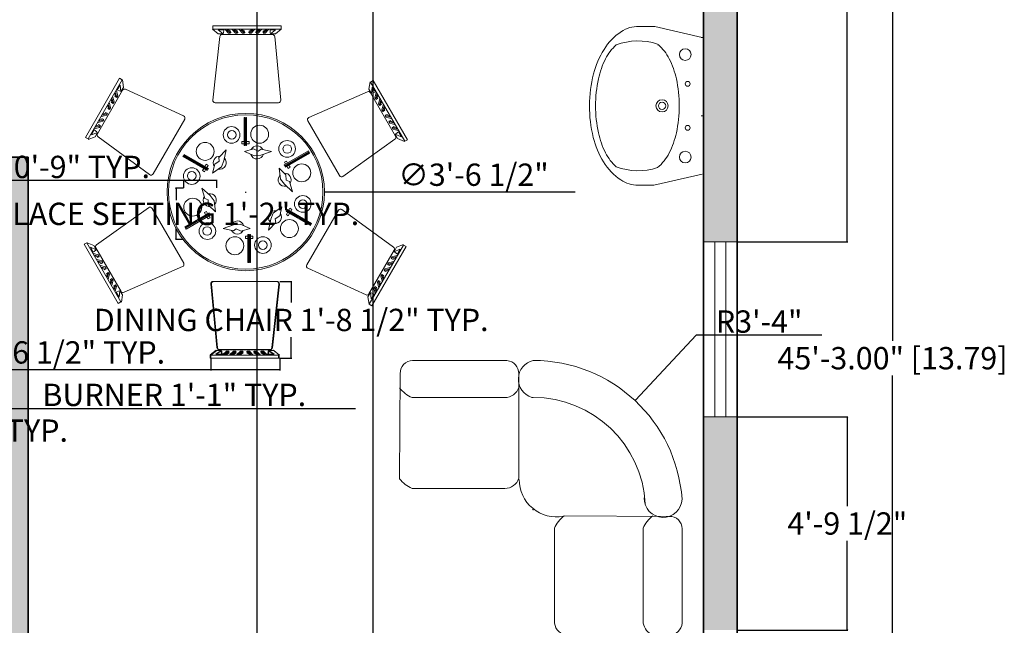
# Model space of a CAD drawing. Units: inches. Extents: x 2322 to 2932, y 142 to 762.
# Tile 6 of 7: x 2609 to 2874, y 376 to 538. Entities that reach past the tile are written whole.
import ezdxf

# ---------------------------------------------------------------- set-up
doc = ezdxf.new("R2010")
doc.units = ezdxf.units.IN
doc.header["$MEASUREMENT"] = 0
for name, color, linetype, lineweight in [('A-ANNO-DIMS', 2, 'Continuous', 18), ('A-FLOR-FIXT', 9, 'Continuous', 18), ('A-GLAZ', 4, 'Continuous', 18), ('A-WALL', 7, 'Continuous', 35)]:
    doc.layers.add(name, color=color, linetype=linetype, lineweight=lineweight)
doc.layers.add('A-WALL-PATT', color=40, linetype='Continuous', lineweight=13, true_color=0xf8d731)
doc.layers.add('Furniture', color=7, linetype='Continuous', lineweight=15, true_color=0xffffff)
doc.styles.get("Standard").update_dxf_attribs({"font": 'italic8.shx'})
doc.dimstyles.get("Standard").update_dxf_attribs({"dimtxt": 6, "dimasz": 0.15, "dimexe": 0.18, "dimexo": 0.0625, "dimgap": 0.09, "dimtad": 1, "dimtih": 1, "dimtoh": 1, "dimzin": 0, "dimdsep": 46, "dimlunit": 3, "dimtxsty": 'Standard', "dimblk": 'CLOSEDBLANK', "dimcen": 0.09, "dimclrd": 3, "dimclre": 1, "dimclrt": 6, "dimadec": 0, "dimazin": 0, "dimtfac": 1, "dimtofl": 0, "dimtmove": 0, "dimatfit": 3, "dimldrblk": 'DOT', "dimfxl": 1, "dimtolj": 1, "dimtzin": 0, "dimarcsym": 0})

# ---------------------------------------------------------------- blocks, each defined once
blk = doc.blocks.new('_ClosedBlank')
at = {"color": 0, "linetype": 'ByBlock', "lineweight": -2}
for p, q in [((-1, 0.2), (0, 0)), ((-1, 0.2), (-1, -0.2)), ((0, 0), (-1, -0.2))]:
    blk.add_line(p, q, dxfattribs=at)
blk = doc.blocks.new('*D3')
at = {"layer": 'A-ANNO-DIMS', "color": 0, "lineweight": -2, "transparency": 16777216}
for p, q in [((2802.13, 718.82), (2844.02, 718.82)), ((2843.84, 718.67), (2843.84, 451.98)), ((2843.84, 175.97), (2843.84, 442.66)), ((2802.13, 175.82), (2844.02, 175.82))]:
    blk.add_line(p, q, dxfattribs=at)
at = {"layer": 'Defpoints', "color": 0, "transparency": 16777216}
for p in [(2802.06, 718.82), (2802.06, 175.82), (2843.84, 175.82)]:
    blk.add_point(p, dxfattribs=at)
at = {"layer": 'A-ANNO-DIMS', "color": 0, "lineweight": -2, "transparency": 16777216, "xscale": 0.15, "yscale": 0.15, "zscale": 0.15}
for p, rotation in [((2843.84, 718.82), 90), ((2843.84, 175.82), 270)]:
    blk.add_blockref('_ClosedBlank', p, dxfattribs=dict(at, rotation=rotation))
at = {"layer": 'A-ANNO-DIMS', "color": 0, "transparency": 16777216, "insert": (2843.84, 447.32), "char_height": 6, "attachment_point": 5}
blk.add_mtext('\\A1;45\'-3.00" [13.79]', dxfattribs=at)
blk = doc.blocks.new('_Dot')
at = {"color": 0, "linetype": 'ByBlock', "lineweight": -2}
blk.add_line((-0.5, 0), (-1, 0), dxfattribs=at)
at = {"color": 0, "linetype": 'ByBlock', "const_width": 0.5}
blk.add_lwpolyline([(-0.25, 0, 1), (0.25, 0, 1)], format="xyb", close=True, dxfattribs=at)
blk = doc.blocks.new('WINDOW-47X9')
for p, q in [((47, 9), (0, 9)), ((0, 9), (0, 0)), ((47, 0), (47, 9)), ((0, 6), (47, 6)), ((0, 3), (47, 3)), ((0, 0), (47, 0))]:
    blk.add_line(p, q)
blk = doc.blocks.new('CHAIR-DINING')
for p, q in [((0, 19.73, 3.57), (1.57, 18.47, 3.57)), ((0.13, 20.61, 3.57), (0.13, 19.79, 3.57)), ((18.48, 20.61, 3.57), (0.13, 20.61, 3.57)), ((0.13, 19.79, 3.57), (18.48, 19.79, 3.57)), ((1.51, 19.54, 3.57), (3.02, 19.6, 3.57)), ((2.89, 18.53, 3.57), (1.51, 19.54, 3.57)), ((1.57, 18.47, 3.57), (2.89, 18.53, 3.57)), ((3.02, 19.6, 3.57), (2.95, 18.72, 3.57)), ((3.39, 19.66, 3.57), (4.34, 18.72, 3.57)), ((3.9, 19.6, 3.57), (4.27, 19.6, 3.57)), ((4.84, 18.72, 3.57), (3.9, 19.6, 3.57)), ((4.27, 19.6, 3.57), (4.71, 19.22, 3.57)), ((4.34, 18.72, 3.57), (4.84, 18.72, 3.57)), ((4.71, 19.22, 3.57), (4.84, 19.35, 3.57)), ((4.84, 19.35, 3.57), (4.9, 18.78, 3.57)), ((5.28, 19.66, 3.57), (6.22, 18.72, 3.57)), ((5.78, 19.6, 3.57), (6.16, 19.6, 3.57)), ((6.73, 18.72, 3.57), (5.78, 19.6, 3.57)), ((6.16, 19.6, 3.57), (6.6, 19.22, 3.57)), ((6.22, 18.72, 3.57), (6.73, 18.72, 3.57)), ((6.6, 19.22, 3.57), (6.73, 19.35, 3.57)), ((6.73, 19.35, 3.57), (6.79, 18.78, 3.57)), ((7.17, 19.66, 3.57), (8.11, 18.72, 3.57)), ((7.67, 19.6, 3.57), (8.05, 19.6, 3.57)), ((8.61, 18.72, 3.57), (7.67, 19.6, 3.57)), ((8.05, 19.6, 3.57), (8.49, 19.22, 3.57)), ((8.11, 18.72, 3.57), (8.61, 18.72, 3.57)), ((8.49, 19.22, 3.57), (8.61, 19.35, 3.57)), ((8.61, 19.35, 3.57), (8.67, 18.78, 3.57)), ((9.87, 19.35, 3.57), (9.81, 18.78, 3.57)), ((9.87, 18.72, 3.57), (10.81, 19.6, 3.57)), ((9.99, 19.22, 3.57), (9.87, 19.35, 3.57)), ((10.37, 18.72, 3.57), (9.87, 18.72, 3.57)), ((10.43, 19.6, 3.57), (9.99, 19.22, 3.57)), ((11.31, 19.66, 3.57), (10.37, 18.72, 3.57)), ((10.81, 19.6, 3.57), (10.43, 19.6, 3.57)), ((11.75, 19.35, 3.57), (11.69, 18.78, 3.57)), ((11.75, 18.72, 3.57), (12.7, 19.6, 3.57)), ((11.88, 19.22, 3.57), (11.75, 19.35, 3.57)), ((12.26, 18.72, 3.57), (11.75, 18.72, 3.57)), ((12.32, 19.6, 3.57), (11.88, 19.22, 3.57)), ((13.2, 19.66, 3.57), (12.26, 18.72, 3.57)), ((12.7, 19.6, 3.57), (12.32, 19.6, 3.57)), ((13.64, 19.35, 3.57), (13.58, 18.78, 3.57)), ((13.64, 18.72, 3.57), (14.58, 19.6, 3.57)), ((13.77, 19.22, 3.57), (13.64, 19.35, 3.57)), ((14.14, 18.72, 3.57), (13.64, 18.72, 3.57)), ((14.21, 19.6, 3.57), (13.77, 19.22, 3.57)), ((15.09, 19.66, 3.57), (14.14, 18.72, 3.57)), ((14.58, 19.6, 3.57), (14.21, 19.6, 3.57)), ((15.46, 19.6, 3.57), (15.53, 18.72, 3.57)), ((16.97, 19.54, 3.57), (15.46, 19.6, 3.57)), ((15.59, 18.53, 3.57), (16.97, 19.54, 3.57)), ((16.91, 18.47, 3.57), (15.59, 18.53, 3.57)), ((18.48, 19.73, 3.57), (16.91, 18.47, 3.57)), ((18.48, 19.79, 3.57), (18.48, 20.61, 3.57)), ((0.08, 0.7, 3.57), (1.95, 17.78, 3.57)), ((2.58, 18.34, 3.57), (16.09, 18.34, 3.57)), ((16.71, 17.78, 3.57), (18.35, 0.69, 3.57)), ((17.72, 0, 3.57), (0.7, 0, 3.57))]:
    blk.add_line(p, q)
for centre, start, end in [((2.58, 17.72, 3.57), 90, 173.7428), ((16.09, 17.72, 3.57), 5.4801, 90), ((0.7, 0.63, 3.57), 173.7428, 270), ((17.72, 0.63, 3.57), 270, 5.4801)]:
    blk.add_arc(centre, 0.629, start, end)
blk = doc.blocks.new('DINING-PLACE-SETTING')
for p, q in [((8.13, 10.96, 7.15), (1.62, 7.2, 7.15)), ((1.74, 6.99, 7.15), (8.25, 10.75, 7.15)), ((8.25, 10.75, 7.15), (8.13, 10.96, 7.15)), ((2.23, 8.25, 7.15), (1.7, 7.95, 7.15)), ((1.7, 7.95, 7.15), (2.01, 7.42, 7.15)), ((8.35, 10.57, 7.15), (1.84, 6.81, 7.15)), ((1.96, 6.61, 7.15), (8.47, 10.37, 7.15)), ((2.54, 7.72, 7.15), (2.23, 8.25, 7.15)), ((8.47, 10.37, 7.15), (8.35, 10.57, 7.15)), ((2.07, 4.55, 7.15), (0.25, 6.3, 7.15)), ((0.25, 6.3, 7.15), (0.59, 3.36, 7.15)), ((1.62, 7.2, 7.15), (1.74, 6.99, 7.15)), ((1.84, 6.81, 7.15), (1.96, 6.61, 7.15)), ((2.12, 7.22, 7.15), (2.23, 7.03, 7.15)), ((2.35, 6.83, 7.15), (2.68, 6.26, 7.15)), ((2.76, 7.34, 7.15), (2.65, 7.52, 7.15)), ((2.68, 6.26, 7.15), (3.21, 6.56, 7.15)), ((3.21, 6.56, 7.15), (2.88, 7.13, 7.15)), ((0.59, 3.36, 7.15), (1.66, 1.99, 7.15)), ((2.19, 3.11, 7.15), (2.07, 4.55, 7.15)), ((3.08, 2.74, 7.15), (2.19, 3.11, 7.15)), ((3.88, 0, 7.15), (3.08, 2.74, 7.15)), ((1.66, 1.99, 7.15), (3.88, 0, 7.15))]:
    blk.add_line(p, q)
for centre, radius in [((2.41, 11.52, 7.15), 2.24), ((2.46, 11.49, 7.15), 1.16), ((6.34, 5.08, 7.15), 2.41)]:
    blk.add_circle(centre, radius)
for start, end in [(137.0611, 284.0662), (326.6641, 94.1442)]:
    blk.add_arc((1.75, 3.22, 7.15), 1.75, start, end)
blk = doc.blocks.new('SECTIONAL-SEAT')
for p, q in [((30.86, 31.9), (2.62, 32.04)), ((0, 28.69), (0, 3.79)), ((23.85, 28.69), (23.85, 3.79)), ((34.36, 3.2), (34.36, 28.55)), ((2.77, 0), (30.86, 0))]:
    blk.add_line(p, q)
for centre, radius, start, end in [((7.53, 25.51), 8.17, 126.8838, 157.0502), ((31.38, 25.51), 8.17, 126.8838, 157.0502), ((31, 28.55), 3.35, 0, 92.4088), ((3.98, 3.79), 3.98, 180, 252.2888), ((27.83, 3.79), 3.98, 180, 244.0743), ((30.86, 3.51), 3.51, 270, 355.0498)]:
    blk.add_arc(centre, radius, start, end)
blk = doc.blocks.new('*D30')
at = {"layer": 'A-ANNO-DIMS', "color": 1, "lineweight": -2, "transparency": 16777216}
for p, q in [((2679.23, 467.9), (2682.44, 467.9)), ((2679.23, 447.3), (2682.44, 447.3))]:
    blk.add_line(p, q, dxfattribs=at)
at = {"layer": 'A-ANNO-DIMS', "color": 3, "lineweight": -2, "transparency": 16777216}
for p, q in [((2682.26, 467.75), (2682.26, 462.26)), ((2682.26, 447.45), (2682.26, 452.94))]:
    blk.add_line(p, q, dxfattribs=at)
at = {"layer": 'Defpoints', "color": 0, "transparency": 16777216}
for p in [(2679.17, 467.9), (2679.17, 447.3), (2682.26, 447.3)]:
    blk.add_point(p, dxfattribs=at)
at = {"layer": 'A-ANNO-DIMS', "color": 3, "lineweight": -2, "transparency": 16777216, "xscale": 0.15, "yscale": 0.15, "zscale": 0.15}
for p, rotation in [((2682.26, 467.9), 90), ((2682.26, 447.3), 270)]:
    blk.add_blockref('_ClosedBlank', p, dxfattribs=dict(at, rotation=rotation))
at = {"layer": 'A-ANNO-DIMS', "color": 6, "transparency": 16777216, "insert": (2682.26, 457.6), "char_height": 6, "attachment_point": 5}
blk.add_mtext('\\A1;DINING CHAIR 1\'-8 1/2" TYP.', dxfattribs=at)
blk = doc.blocks.new('*D31')
at = {"layer": 'A-ANNO-DIMS', "color": 1, "lineweight": -2, "transparency": 16777216}
for p, q in [((2660.69, 447.24), (2660.69, 444.03)), ((2679.17, 447.24), (2679.17, 444.03))]:
    blk.add_line(p, q, dxfattribs=at)
at = {"layer": 'A-ANNO-DIMS', "color": 3, "lineweight": -2, "transparency": 16777216}
for p, q in [((2660.69, 444.21), (2585.5, 444.21)), ((2679.02, 444.21), (2660.84, 444.21))]:
    blk.add_line(p, q, dxfattribs=at)
at = {"layer": 'Defpoints', "color": 0, "transparency": 16777216}
for p in [(2660.69, 447.3), (2679.17, 447.3), (2660.69, 444.21)]:
    blk.add_point(p, dxfattribs=at)
at = {"layer": 'A-ANNO-DIMS', "color": 3, "lineweight": -2, "transparency": 16777216, "xscale": 0.15, "yscale": 0.15, "zscale": 0.15, "rotation": 180}
blk.add_blockref('_ClosedBlank', (2660.69, 444.21), dxfattribs=at)
at = {"layer": 'A-ANNO-DIMS', "color": 3, "lineweight": -2, "transparency": 16777216, "xscale": 0.15, "yscale": 0.15, "zscale": 0.15}
blk.add_blockref('_ClosedBlank', (2679.17, 444.21), dxfattribs=at)
at = {"layer": 'A-ANNO-DIMS', "color": 6, "transparency": 16777216, "insert": (2623.02, 448.87), "char_height": 6, "attachment_point": 5}
blk.add_mtext('\\A1;1\'-6 1/2" TYP.', dxfattribs=at)
blk = doc.blocks.new('*D32')
at = {"layer": 'A-ANNO-DIMS', "color": 1, "lineweight": -2, "transparency": 16777216}
for p, q in [((2653.34, 493), (2651.16, 493)), ((2653.34, 479.24), (2651.16, 479.24))]:
    blk.add_line(p, q, dxfattribs=at)
at = {"layer": 'A-ANNO-DIMS', "color": 3, "lineweight": -2, "transparency": 16777216}
for p, q in [((2651.34, 492.85), (2651.34, 489.78)), ((2651.34, 479.39), (2651.34, 482.46))]:
    blk.add_line(p, q, dxfattribs=at)
at = {"layer": 'Defpoints', "color": 0, "transparency": 16777216}
for p in [(2653.4, 493), (2651.34, 479.24), (2653.4, 479.24)]:
    blk.add_point(p, dxfattribs=at)
at = {"layer": 'A-ANNO-DIMS', "color": 3, "lineweight": -2, "transparency": 16777216, "xscale": 0.15, "yscale": 0.15, "zscale": 0.15}
for p, rotation in [((2651.34, 493), 90), ((2651.34, 479.24), 270)]:
    blk.add_blockref('_ClosedBlank', p, dxfattribs=dict(at, rotation=rotation))
at = {"layer": 'A-ANNO-DIMS', "color": 6, "transparency": 16777216, "insert": (2651.34, 486.12), "char_height": 6, "attachment_point": 5}
blk.add_mtext('\\A1;PLACE SETTING 1\'-2" TYP.', dxfattribs=at)
blk = doc.blocks.new('*D33')
at = {"layer": 'A-ANNO-DIMS', "color": 3, "lineweight": -2, "transparency": 16777216}
for p, q in [((2653.4, 495.07), (2598.79, 495.07)), ((2662.16, 495.07), (2653.55, 495.07))]:
    blk.add_line(p, q, dxfattribs=at)
at = {"layer": 'A-ANNO-DIMS', "color": 1, "lineweight": -2, "transparency": 16777216}
for p, q in [((2653.4, 493.07), (2653.4, 495.25)), ((2662.31, 493.07), (2662.31, 495.25))]:
    blk.add_line(p, q, dxfattribs=at)
at = {"layer": 'Defpoints', "color": 0, "transparency": 16777216}
for p in [(2653.4, 495.07), (2653.4, 493), (2662.31, 493)]:
    blk.add_point(p, dxfattribs=at)
at = {"layer": 'A-ANNO-DIMS', "color": 3, "lineweight": -2, "transparency": 16777216, "xscale": 0.15, "yscale": 0.15, "zscale": 0.15, "rotation": 180}
blk.add_blockref('_ClosedBlank', (2653.4, 495.07), dxfattribs=at)
at = {"layer": 'A-ANNO-DIMS', "color": 3, "lineweight": -2, "transparency": 16777216, "xscale": 0.15, "yscale": 0.15, "zscale": 0.15}
blk.add_blockref('_ClosedBlank', (2662.31, 495.07), dxfattribs=at)
at = {"layer": 'A-ANNO-DIMS', "color": 6, "transparency": 16777216, "insert": (2626.02, 498.73), "char_height": 6, "attachment_point": 5}
blk.add_mtext('\\A1;0\'-9" TYP.', dxfattribs=at)
blk = doc.blocks.new('*D42')
at = {"layer": 'A-ANNO-DIMS', "color": 1, "lineweight": -2, "transparency": 16777216}
for p, q in [((2589.15, 431.92), (2589.15, 433.98)), ((2602.04, 431.92), (2602.04, 433.98))]:
    blk.add_line(p, q, dxfattribs=at)
at = {"layer": 'A-ANNO-DIMS', "color": 3, "lineweight": -2, "transparency": 16777216}
for p, q in [((2589.3, 433.8), (2601.89, 433.8)), ((2602.04, 433.8), (2699.51, 433.8))]:
    blk.add_line(p, q, dxfattribs=at)
at = {"layer": 'Defpoints', "color": 0, "transparency": 16777216}
for p in [(2589.15, 431.86), (2602.04, 433.8), (2602.04, 431.86)]:
    blk.add_point(p, dxfattribs=at)
at = {"layer": 'A-ANNO-DIMS', "color": 3, "lineweight": -2, "transparency": 16777216, "xscale": 0.15, "yscale": 0.15, "zscale": 0.15, "rotation": 180}
blk.add_blockref('_ClosedBlank', (2589.15, 433.8), dxfattribs=at)
at = {"layer": 'A-ANNO-DIMS', "color": 3, "lineweight": -2, "transparency": 16777216, "xscale": 0.15, "yscale": 0.15, "zscale": 0.15}
blk.add_blockref('_ClosedBlank', (2602.04, 433.8), dxfattribs=at)
at = {"layer": 'A-ANNO-DIMS', "color": 6, "transparency": 16777216, "insert": (2650.85, 437.46), "char_height": 6, "attachment_point": 5}
blk.add_mtext('\\A1;BURNER 1\'-1" TYP.', dxfattribs=at)
blk = doc.blocks.new('*D43')
at = {"layer": 'A-ANNO-DIMS', "color": 1, "lineweight": -2, "transparency": 16777216}
for p, q in [((2602.1, 431.86), (2604.15, 431.86)), ((2602.1, 423.83), (2604.15, 423.83))]:
    blk.add_line(p, q, dxfattribs=at)
at = {"layer": 'A-ANNO-DIMS', "color": 3, "lineweight": -2, "transparency": 16777216}
for p, q in [((2603.97, 431.71), (2603.97, 431.51)), ((2603.97, 423.98), (2603.97, 424.19))]:
    blk.add_line(p, q, dxfattribs=at)
at = {"layer": 'Defpoints', "color": 0, "transparency": 16777216}
for p in [(2602.04, 431.86), (2602.04, 423.83), (2603.97, 423.83)]:
    blk.add_point(p, dxfattribs=at)
at = {"layer": 'A-ANNO-DIMS', "color": 3, "lineweight": -2, "transparency": 16777216, "xscale": 0.15, "yscale": 0.15, "zscale": 0.15}
for p, rotation in [((2603.97, 431.86), 90), ((2603.97, 423.83), 270)]:
    blk.add_blockref('_ClosedBlank', p, dxfattribs=dict(at, rotation=rotation))
at = {"layer": 'A-ANNO-DIMS', "color": 6, "transparency": 16777216, "insert": (2603.97, 427.85), "char_height": 6, "attachment_point": 5}
blk.add_mtext('\\A1;0\'-8" TYP.', dxfattribs=at)
blk = doc.blocks.new('*D54')
at = {"layer": 'A-ANNO-DIMS', "color": 1, "lineweight": -2, "transparency": 16777216}
for p, q in [((2673.06, 709.76), (2673.06, 146.01)), ((2704.23, 709.76), (2704.23, 146.01))]:
    blk.add_line(p, q, dxfattribs=at)
at = {"layer": 'A-ANNO-DIMS', "color": 3, "lineweight": -2, "transparency": 16777216}
blk.add_line((2673.21, 146.19), (2704.08, 146.19), dxfattribs=at)
at = {"layer": 'Defpoints', "color": 0, "transparency": 16777216}
for p in [(2673.06, 709.82), (2704.23, 709.82), (2704.23, 146.19)]:
    blk.add_point(p, dxfattribs=at)
at = {"layer": 'A-ANNO-DIMS', "color": 3, "lineweight": -2, "transparency": 16777216, "xscale": 0.15, "yscale": 0.15, "zscale": 0.15, "rotation": 180}
blk.add_blockref('_ClosedBlank', (2673.06, 146.19), dxfattribs=at)
at = {"layer": 'A-ANNO-DIMS', "color": 3, "lineweight": -2, "transparency": 16777216, "xscale": 0.15, "yscale": 0.15, "zscale": 0.15}
blk.add_blockref('_ClosedBlank', (2704.23, 146.19), dxfattribs=at)
at = {"layer": 'A-ANNO-DIMS', "color": 6, "transparency": 16777216, "insert": (2688.65, 149.85), "char_height": 6, "attachment_point": 5}
blk.add_mtext('\\A1;2\'-7"', dxfattribs=at)
blk = doc.blocks.new('*D63')
at = {"layer": 'A-ANNO-DIMS', "color": 1, "lineweight": -2, "transparency": 16777216}
for p, q in [((2802.13, 431.57), (2831.87, 431.57)), ((2802.13, 374.22), (2831.87, 374.22))]:
    blk.add_line(p, q, dxfattribs=at)
at = {"layer": 'A-ANNO-DIMS', "color": 3, "lineweight": -2, "transparency": 16777216}
for p, q in [((2831.69, 431.42), (2831.69, 407.55)), ((2831.69, 374.37), (2831.69, 398.23))]:
    blk.add_line(p, q, dxfattribs=at)
at = {"layer": 'Defpoints', "color": 0, "transparency": 16777216}
for p in [(2802.06, 431.57), (2831.69, 431.57), (2802.06, 374.22)]:
    blk.add_point(p, dxfattribs=at)
at = {"layer": 'A-ANNO-DIMS', "color": 3, "lineweight": -2, "transparency": 16777216, "xscale": 0.15, "yscale": 0.15, "zscale": 0.15}
for p, rotation in [((2831.69, 431.57), 90), ((2831.69, 374.22), 270)]:
    blk.add_blockref('_ClosedBlank', p, dxfattribs=dict(at, rotation=rotation))
at = {"layer": 'A-ANNO-DIMS', "color": 6, "transparency": 16777216, "insert": (2831.69, 402.89), "char_height": 6, "attachment_point": 5}
blk.add_mtext('\\A1;4\'-9 1/2"', dxfattribs=at)
blk = doc.blocks.new('*D64')
at = {"layer": 'A-ANNO-DIMS', "color": 1, "lineweight": -2, "transparency": 16777216}
for p, q in [((2802.13, 613.14), (2831.87, 613.14)), ((2802.13, 478.57), (2831.87, 478.57))]:
    blk.add_line(p, q, dxfattribs=at)
at = {"layer": 'A-ANNO-DIMS', "color": 3, "lineweight": -2, "transparency": 16777216}
for p, q in [((2831.69, 612.99), (2831.69, 550.51)), ((2831.69, 478.72), (2831.69, 541.19))]:
    blk.add_line(p, q, dxfattribs=at)
at = {"layer": 'Defpoints', "color": 0, "transparency": 16777216}
for p in [(2802.06, 613.14), (2831.69, 613.14), (2802.06, 478.57)]:
    blk.add_point(p, dxfattribs=at)
at = {"layer": 'A-ANNO-DIMS', "color": 3, "lineweight": -2, "transparency": 16777216, "xscale": 0.15, "yscale": 0.15, "zscale": 0.15}
for p, rotation in [((2831.69, 613.14), 90), ((2831.69, 478.57), 270)]:
    blk.add_blockref('_ClosedBlank', p, dxfattribs=dict(at, rotation=rotation))
at = {"layer": 'A-ANNO-DIMS', "color": 6, "transparency": 16777216, "insert": (2831.69, 545.85), "char_height": 6, "attachment_point": 5}
blk.add_mtext('\\A1;11\'-2 1/2"', dxfattribs=at)
blk = doc.blocks.new('*D66')
at = {"layer": 'A-ANNO-DIMS', "color": 1, "lineweight": -2, "transparency": 16777216}
for p, q in [((2669.97, 491.98), (2670.15, 491.98)), ((2670.06, 491.89), (2670.06, 492.07))]:
    blk.add_line(p, q, dxfattribs=at)
at = {"layer": 'A-ANNO-DIMS', "color": 3, "lineweight": -2, "transparency": 16777216}
for p, q in [((2703.89, 491.98), (2691.35, 491.98)), ((2758.55, 491.98), (2703.89, 491.98))]:
    blk.add_line(p, q, dxfattribs=at)
at = {"layer": 'Defpoints', "color": 0, "transparency": 16777216}
for p in [(2648.92, 491.98), (2691.2, 491.98)]:
    blk.add_point(p, dxfattribs=at)
at = {"layer": 'A-ANNO-DIMS', "color": 3, "lineweight": -2, "transparency": 16777216, "xscale": 0.15, "yscale": 0.15, "zscale": 0.15, "rotation": 179.9988401368386}
blk.add_blockref('_ClosedBlank', (2691.2, 491.98), dxfattribs=at)
at = {"layer": 'A-ANNO-DIMS', "color": 6, "transparency": 16777216, "insert": (2731.26, 496.64), "char_height": 6, "attachment_point": 5}
blk.add_mtext('\\A1;∅3\'-6 1/2"', dxfattribs=at)
blk = doc.blocks.new('*D67')
at = {"layer": 'A-ANNO-DIMS', "color": 3, "lineweight": -2, "transparency": 16777216}
for p, q in [((2791.06, 453.51), (2774.75, 436.04)), ((2824.87, 453.51), (2791.06, 453.51))]:
    blk.add_line(p, q, dxfattribs=at)
at = {"layer": 'A-ANNO-DIMS', "color": 1, "lineweight": -2, "transparency": 16777216}
for p, q in [((2747.2, 406.62), (2747.38, 406.62)), ((2747.29, 406.53), (2747.29, 406.71))]:
    blk.add_line(p, q, dxfattribs=at)
at = {"layer": 'Defpoints', "color": 0, "transparency": 16777216}
for p in [(2774.65, 435.93), (2747.29, 406.62)]:
    blk.add_point(p, dxfattribs=at)
at = {"layer": 'A-ANNO-DIMS', "color": 3, "lineweight": -2, "transparency": 16777216, "xscale": 0.15, "yscale": 0.15, "zscale": 0.15, "rotation": 226.9669669756744}
blk.add_blockref('_ClosedBlank', (2774.65, 435.93), dxfattribs=at)
at = {"layer": 'A-ANNO-DIMS', "color": 6, "transparency": 16777216, "insert": (2808.01, 457.17), "char_height": 6, "attachment_point": 5}
blk.add_mtext('\\A1;R3\'-4"', dxfattribs=at)

msp = doc.modelspace()

# ---------------------------------------------------------------- hatches: boundary and pattern name
at = {"layer": 'A-WALL-PATT'}
h = msp.add_hatch(color=256, dxfattribs=at)
h.dxf.hatch_style = 1
h.paths.add_polyline_path([(2439.065, 709.819), (2491.097, 709.819), (2491.097, 718.819), (2430.065, 718.819), (2430.065, 663.548), (2439.065, 663.548)])
h.paths.add_polyline_path([(2704.233, 718.819), (2654.246, 718.819), (2654.246, 709.819), (2668.565, 709.819), (2668.565, 661.819), (2673.065, 661.819), (2673.065, 709.819), (2704.233, 709.819)], flags=17)
h.paths.add_polyline_path([(2624.246, 718.819), (2538.097, 718.819), (2538.097, 709.819), (2607.065, 709.819), (2607.065, 565.819), (2583.065, 565.819), (2583.065, 561.319), (2611.565, 561.319), (2611.565, 609.319), (2668.565, 609.319), (2668.565, 561.319), (2758.065, 561.319), (2758.065, 565.819), (2673.065, 565.819), (2673.065, 626.819), (2668.565, 626.819), (2668.565, 613.819), (2611.565, 613.819), (2611.565, 709.819), (2624.246, 709.819)])
h.paths.add_polyline_path([(2802.065, 718.819), (2751.233, 718.819), (2751.233, 709.819), (2793.065, 709.819), (2793.065, 660.138), (2802.065, 660.138)])
h.paths.add_polyline_path([(2802.065, 613.138), (2793.065, 613.138), (2793.065, 478.568), (2802.065, 478.568)])
h.paths.add_polyline_path([(2439.065, 616.548), (2430.065, 616.548), (2430.065, 551.562), (2439.065, 551.562), (2439.065, 561.319), (2483.455, 561.319), (2483.455, 565.819), (2439.065, 565.819)])
h.paths.add_polyline_path([(2548.065, 565.819), (2518.455, 565.819), (2518.455, 561.319), (2541.065, 561.319), (2541.065, 501.319), (2439.065, 501.319), (2439.065, 516.562), (2430.065, 516.562), (2430.065, 465.181), (2439.065, 465.181), (2439.065, 496.819), (2503.266, 496.819), (2541.065, 496.819), (2541.065, 472.819), (2545.565, 472.819), (2545.565, 561.319), (2548.065, 561.319)])
h.paths.add_polyline_path([(2439.065, 418.181), (2430.065, 418.181), (2430.065, 342.453), (2439.065, 342.453), (2439.065, 367.819), (2602.565, 367.819), (2602.565, 283.756), (2594.693, 283.756), (2594.693, 274.756), (2611.565, 274.756), (2611.565, 501.319), (2580.942, 501.319), (2580.942, 496.819), (2607.065, 496.819), (2607.065, 376.819), (2439.065, 376.819)])
h.paths.add_polyline_path([(2793.057, 530.805), (2793.057, 530.68), (2793.106, 530.68), (2793.106, 530.805)], flags=25)
h.paths.add_polyline_path([(2793.057, 530.808), (2793.057, 530.676), (2793.106, 530.676), (2793.106, 530.808)], flags=9)
h = msp.add_hatch(color=256, dxfattribs=at)
h.dxf.hatch_style = 1
h.paths.add_polyline_path([(2559.693, 283.756), (2439.065, 283.756), (2439.065, 295.453), (2430.065, 295.453), (2430.065, 274.756), (2559.693, 274.756)])
h.paths.add_polyline_path([(2802.065, 431.568), (2793.065, 431.568), (2793.065, 374.218), (2802.065, 374.218)])
h.paths.add_polyline_path([(2802.065, 327.218), (2793.065, 327.218), (2793.065, 283.756), (2708.065, 283.756), (2708.065, 279.256), (2793.065, 279.256), (2793.065, 260.879), (2802.065, 260.879)])
h.paths.add_polyline_path([(2673.065, 283.756), (2664.065, 283.756), (2664.065, 175.819), (2710.255, 175.819), (2710.255, 184.819), (2673.065, 184.819)])
h.paths.add_polyline_path([(2802.065, 213.879), (2793.065, 213.879), (2793.065, 184.819), (2757.255, 184.819), (2757.255, 175.819), (2802.065, 175.819)])

# ---------------------------------------------------------------- linework, layer by layer
at = {"layer": 'A-FLOR-FIXT'}
for p, q in [((2779.704, 536.52), (2775.464, 536.521)), ((2779.978, 536.516), (2792.737, 533.521)), ((2792.409, 533.521), (2793.065, 533.521)), ((2793.065, 533.521), (2793.065, 496.787)), ((2780.673, 531.586), (2780.885, 531.586)), ((2781.071, 531.408), (2780.934, 531.564)), ((2793.065, 512.441), (2792.409, 512.441)), ((2779.704, 493.788), (2792.737, 496.787)), ((2779.704, 493.788), (2775.464, 493.787))]:
    msp.add_line(p, q, dxfattribs=at)
for centre, radius in [((2788.145, 528.929), 1.574), ((2788.145, 528.929), 1.574), ((2788.145, 528.929), 1.574), ((2788.801, 521.058), 0.656), ((2781.913, 515.154), 1.64), ((2781.913, 515.154), 0.984), ((2788.801, 509.251), 0.656), ((2788.145, 501.379), 1.574)]:
    msp.add_circle(centre, radius, dxfattribs=at)
for centre, radius, start, end in [((2779.775, 521.951), 15.835, 123.73047, 148.17791), ((2775.603, 528.199), 8.322, 89.76763, 123.73047), ((2779.67, 528.199), 8.322, 87.88301, 89.76763), ((2775.469, 516.041), 16.565, 71.53867, 110.69778), ((2786.448, 517.81), 23.688, 148.17791, 165.47696), ((2778.208, 521.943), 12.88, 131.94987, 152.8258), ((2772.368, 521.943), 12.88, 27.1742, 48.62612), ((2780.885, 531.521), 0.0656, 41.32236, 90), ((2786.182, 517.85), 21.843, 152.8258, 167.99536), ((2764.395, 517.85), 21.843, 12.00464, 27.1742), ((2797.038, 515.067), 34.627, 165.47696, 179.76763), ((2798.858, 515.154), 34.803, 167.99536, 180), ((2751.718, 515.154), 34.803, 0, 12.00464), ((2797.038, 515.067), 34.627, 179.76763, 194.0583), ((2798.858, 515.154), 34.803, 180, 192.00464), ((2751.718, 515.154), 34.803, 347.99536, 0), ((2786.426, 512.41), 23.688, 194.0583, 211.35734), ((2786.182, 512.459), 21.843, 192.00464, 207.1742), ((2764.395, 512.459), 21.843, 332.8258, 347.99536), ((2779.72, 508.323), 15.835, 211.35734, 235.80478), ((2778.208, 508.365), 12.88, 207.1742, 228.14439), ((2772.368, 508.365), 12.88, 310.39006, 332.8258), ((2775.469, 514.268), 16.565, 249.30222, 288.46133), ((2775.498, 502.109), 8.322, 235.80478, 269.76763), ((2775.498, 502.109), 8.322, 269.76763, 270.96062)]:
    msp.add_arc(centre, radius, start, end, dxfattribs=at)
at = {"layer": 'A-WALL'}
for p, q in [((2802.065, 175.819), (2802.065, 718.819)), ((2793.065, 283.756), (2793.065, 709.819)), ((2611.565, 501.319), (2580.942, 501.319)), ((2611.565, 501.319), (2611.565, 274.756))]:
    msp.add_line(p, q, dxfattribs=at)
at = {"layer": 'Furniture'}
for p, q in [((2740.246, 446.666), (2714.903, 446.666)), ((2711.407, 414.929), (2711.553, 443.172)), ((2743.451, 415.075), (2743.451, 443.172)), ((2743.451, 439.488), (2743.451, 439.588)), ((2714.757, 436.722), (2739.664, 436.722)), ((2746.951, 436.772), (2747.292, 436.772)), ((2714.757, 412.309), (2739.664, 412.309))]:
    msp.add_line(p, q, dxfattribs=at)
for radius in [21.143, 20.749]:
    msp.add_circle((2670.06, 491.983, 3.573), radius, dxfattribs=at)
for centre, radius, start, end in [((2714.903, 443.313), 3.353, 90, 182.40882), ((2739.944, 443.172), 3.507, 0, 85.04975), ((2748.434, 441.692), 5.139, 102.42608, 253.23349), ((2747.292, 406.624), 40.087, 3.98704, 89.94828), ((2717.943, 444.247), 8.172, 216.8838, 247.05023), ((2739.664, 440.697), 3.975, 270, 342.28877), ((2747.292, 406.624), 30.148, 2.91594, 90), ((2717.943, 419.834), 8.172, 216.8838, 247.05023), ((2739.664, 416.284), 3.975, 270, 342.28877), ((2753.569, 414.707), 10.046, 180, 280.60062), ((2782.207, 409.608), 5.079, 178.01213, 358.01213)]:
    msp.add_arc(centre, radius, start, end, dxfattribs=at)

# ---------------------------------------------------------------- block references
at = {"layer": 'A-GLAZ', "rotation": 89.9999999999987}
msp.add_blockref('WINDOW-47X9', (2802.064, 431.568), dxfattribs=at)
at = {"layer": 'Furniture'}
for name, p in [('CHAIR-DINING', (2661.116, 516.004)), ('DINING-PLACE-SETTING', (2678.765, 492.065)), ('SECTIONAL-SEAT', (2752.972, 372.904))]:
    msp.add_blockref(name, p, dxfattribs=at)
for name, p, rotation in [('CHAIR-DINING', (2644.786, 496.248), 59.99999999999815), ('CHAIR-DINING', (2686.391, 511.74), 300.0000000000011), ('DINING-PLACE-SETTING', (2675.019, 499.491), 59.99999999997967), ('DINING-PLACE-SETTING', (2666.715, 499.96), 119.9999999999947), ('DINING-PLACE-SETTING', (2662.157, 493.003), 180), ('DINING-PLACE-SETTING', (2674.207, 485.108), 300.000000000002), ('CHAIR-DINING', (2653.73, 472.227), 120.0000000000024), ('CHAIR-DINING', (2695.335, 487.719), 239.9999999999989), ('DINING-PLACE-SETTING', (2665.903, 485.577), 240.000000000003), ('CHAIR-DINING', (2679.004, 467.963), 180), ('CHAIR-DINING', (2679.167, 467.903), 180)]:
    msp.add_blockref(name, p, dxfattribs=dict(at, rotation=rotation))

# ---------------------------------------------------------------- texts
at = {"layer": 'A-FLOR-FIXT', "width": 0.8, "flags": 9}
for tag, s in [('XSIZE', '650'), ('YSIZE', '450')]:
    msp.add_attdef(tag, (2793.065, 530.808), s, height=0.0328, rotation=270, dxfattribs=at)

# ---------------------------------------------------------------- dimensions: what is measured, and where the dimension line sits
at = {"layer": 'A-ANNO-DIMS'}
for base, p1, p2, override, picture, middle in [((2843.838, 175.819), (2802.065, 718.819), (2802.065, 175.819), {"dimclrd": 0, "dimclre": 0, "dimclrt": 0}, '*D3', (2843.838, 447.319)), ((2831.69, 613.138), (2802.065, 478.568), (2802.065, 613.138), {"dimdec": 1, "dimlfac": 1, "dimrnd": 0, "dimzin": 1, "dimdsep": 46, "dimlunit": 4, "dimfrac": 2}, '*D64', (2831.69, 545.853)), ((2831.6897, 431.5681), (2802.0647, 374.2184), (2802.0647, 431.5681), {"dimdec": 1, "dimlfac": 1, "dimrnd": 0, "dimzin": 1, "dimdsep": 46, "dimlunit": 4, "dimfrac": 2}, '*D63', (2831.6897, 402.8932))]:
    dim = msp.add_linear_dim(base=base, p1=p1, p2=p2, angle=90, dimstyle='Standard', override=override, dxfattribs=at)
    dim.commit()
    dim.dimension.update_dxf_attribs({"geometry": picture, "text_midpoint": middle})
dim = msp.add_linear_dim(base=(2704.233, 146.194), p1=(2673.065, 709.819), p2=(2704.233, 709.819), dimstyle='Standard', override={"dimdec": 1, "dimlfac": 1, "dimrnd": 0, "dimzin": 1, "dimdsep": 46, "dimlunit": 4, "dimfrac": 2}, dxfattribs=at)
dim.commit()
dim.dimension.update_dxf_attribs({"geometry": '*D54', "text_midpoint": (2688.649, 149.855)})
for base, p1, p2, angle, text, picture, middle in [((2653.405, 495.067), (2662.308, 493.003), (2653.405, 493.003), 180, '<> TYP.', '*D33', (2626.022, 498.729)), ((2651.341, 479.242), (2653.405, 493.003), (2653.405, 479.242), 270, 'PLACE SETTING <> TYP.', '*D32', (2651.341, 486.122)), ((2682.257, 447.298), (2679.166, 467.903), (2679.166, 447.298), 270, 'DINING CHAIR <> TYP.', '*D30', (2682.257, 457.601)), ((2660.687, 444.207), (2679.166, 447.298), (2660.687, 447.298), 180, '<> TYP.', '*D31', (2623.019, 448.868)), ((2603.969, 423.833), (2602.036, 431.862), (2602.036, 423.833), 270, '<> TYP.', '*D43', (2603.969, 427.848))]:
    dim = msp.add_linear_dim(base=base, p1=p1, p2=p2, angle=angle, text=text, dimstyle='Standard', override={"dimdec": 1, "dimlfac": 1, "dimrnd": 0, "dimzin": 1, "dimdsep": 46, "dimlunit": 4, "dimfrac": 2}, dxfattribs=at)
    dim.commit()
    dim.dimension.update_dxf_attribs({"geometry": picture, "text_midpoint": middle})
dim = msp.add_diameter_dim_2p(p1=(2648.918, 491.984), p2=(2691.203, 491.983), dimstyle='Standard', override={"dimdec": 1, "dimlfac": 1, "dimrnd": 0, "dimzin": 1, "dimdsep": 46, "dimlunit": 4, "dimfrac": 2}, dxfattribs=at)
dim.commit()
dim.dimension.update_dxf_attribs({"geometry": '*D66', "text_midpoint": (2703.888, 491.983), "dimtype": 163})
dim = msp.add_radius_dim(center=(2747.292, 406.624), mpoint=(2774.648, 435.926), dimstyle='Standard', override={"dimdec": 1, "dimlfac": 1, "dimrnd": 0, "dimzin": 1, "dimdsep": 46, "dimlunit": 4, "dimfrac": 2}, dxfattribs=at)
dim.commit()
dim.dimension.update_dxf_attribs({"geometry": '*D67', "text_midpoint": (2808.009, 453.507), "dimtype": 164})
dim = msp.add_linear_dim(base=(2602.036, 433.795), p1=(2589.149, 431.862), p2=(2602.036, 431.862), text='BURNER <> TYP.', dimstyle='Standard', override={"dimdec": 1, "dimlfac": 1, "dimrnd": 0, "dimzin": 1, "dimdsep": 46, "dimlunit": 4, "dimfrac": 2}, dxfattribs=at)
dim.commit()
dim.dimension.update_dxf_attribs({"geometry": '*D42', "text_midpoint": (2650.847, 437.457)})

doc.saveas('drawing.dxf')
